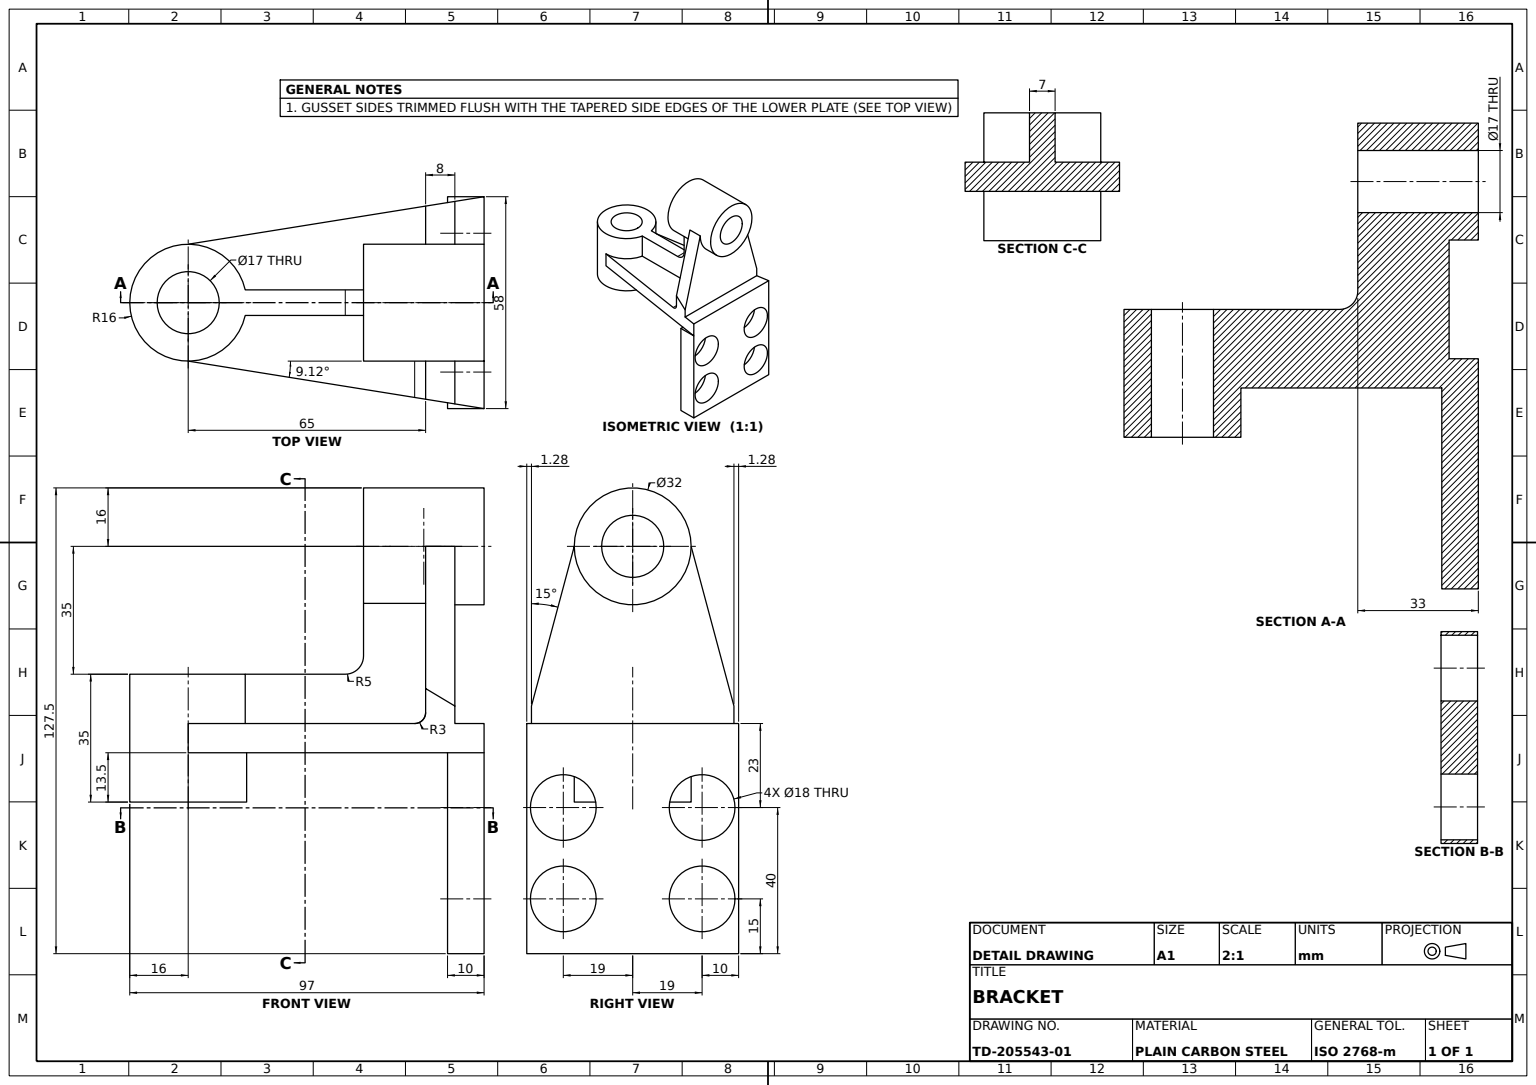
from build123d import *

# Parameters (mm, degrees)
MAIN_BOSS_SKETCH_32_R    = 16
MAIN_BOSS_32_DEPTH       = 17.5
MAIN_BOSS_BORE_SKETCH_R  = 8.5
MAIN_BOSS_BORE_DEPTH     = 57
LOWER_ARM_PLATE_DEPTH    = 4
UPPER_BOSS_SKETCH_R      = 16
UPPER_BOSS_DEPTH         = 33
UPPER_BOSS_BORE_SKETCH_R = 8.5
UPPER_BOSS_BORE_DEPTH    = 38
UPPER_ARM_PLATE_DEPTH    = 8
PLATE_CUT_SET_A_DEPTH    = 38
PLATE_CUT_SET_B_DEPTH    = 38
RIB_DEPTH                = 3.5
RIB_FILLET_R5_R          = 5
ARM_JUNCTION_FILLET_R3_R = 3
GUSSET_SKETCH_W          = 58
GUSSET_SKETCH_H          = 10
GUSSET_DEPTH             = 55
GUSSET_TRIM_SKETCH_R     = 9
GUSSET_TRIM_CUT_DEPTH    = 55


with BuildPart() as part:
    # Main Boss Sketch Ø32 → Main Boss Ø32 (new, symmetric)
    with BuildSketch(Plane(origin=(0, 0, 0), x_dir=(1, 0, 0), z_dir=(0, 1, 0))):
        with Locations(Location((0, 0, 0), (0, 0, 270))):
            Circle(MAIN_BOSS_SKETCH_32_R)
    extrude(amount=MAIN_BOSS_32_DEPTH, both=True)

    # Main Boss Bore Sketch → Main Boss Bore (cut)
    with BuildSketch(Plane(origin=(0, 17.5, 0), x_dir=(1, 0, 0), z_dir=(0, 1, 0))):
        with Locations(Location((0, 0, 0), (0, 0, 270))):
            Circle(MAIN_BOSS_BORE_SKETCH_R)
    extrude(amount=-MAIN_BOSS_BORE_DEPTH, mode=Mode.SUBTRACT)

    # Lower Arm Sketch → Lower Arm Plate (add, symmetric)
    with BuildSketch(Plane(origin=(0, 0, 0), x_dir=(1, 0, 0), z_dir=(0, 1, 0))):
        with BuildLine():
            Line((0, 81), (29, 81))
            Line((29, 81), (16, 0))
            ThreePointArc((16, 0), (0, 16), (-16, 0))
            Line((-16, 0), (-29, 81))
            Line((-29, 81), (0, 81))
        make_face()
    extrude(amount=LOWER_ARM_PLATE_DEPTH, both=True)



with BuildPart() as body_2:
    # Upper Boss Sketch → Upper Boss (new body)
    with BuildSketch(Plane.XY.offset(-48)):
        with Locations((0, 52.5)):
            Circle(UPPER_BOSS_SKETCH_R)
    extrude(amount=-UPPER_BOSS_DEPTH)

    # Upper Boss Bore Sketch → Upper Boss Bore (cut)
    with BuildSketch(Plane.XY.offset(-48)):
        with Locations((0, 52.5)):
            Circle(UPPER_BOSS_BORE_SKETCH_R)
    extrude(amount=-UPPER_BOSS_BORE_DEPTH, mode=Mode.SUBTRACT)


with BuildPart() as part_1:
    add(part.part)

    add(body_2.part)  # Upper Arm Plate merges body 2
    # Upper Arm Sketch → Upper Arm Plate (add)
    with BuildSketch(Plane.XY.offset(-65)):
        with BuildLine():
            Line((-26.431737368, 4), (29, 4))
            Line((29, 4), (16, 52.5))
            ThreePointArc((16, 52.5), (0, 36.5), (-16, 52.5))
            Line((-16, 52.5), (-29, 4))
            Line((-29, 4), (-26.431737368, 4))
        make_face()
    extrude(amount=-UPPER_ARM_PLATE_DEPTH)

    # Plate Cut Set A Sketch → Plate Cut Set A (cut)
    with BuildSketch(Plane.XZ.offset(4)):
        Polygon((27.716049383, -73), (26.432098765, -65), (29, -65), (29, -73), align=None)
    extrude(amount=-PLATE_CUT_SET_A_DEPTH, mode=Mode.SUBTRACT)

    # Plate Cut Set B Sketch → Plate Cut Set B (cut)
    with BuildSketch(Plane.XZ.offset(4)):
        Polygon((-26.432098765, -65), (-29, -65), (-29, -73), (-27.716049383, -73), align=None)
    extrude(amount=-PLATE_CUT_SET_B_DEPTH, mode=Mode.SUBTRACT)

    # Rib Sketch → Rib (add, symmetric)
    with BuildSketch(Plane(origin=(0, 0, 0), x_dir=(0, 0, -1), z_dir=(1, 0, 0))):
        Polygon((48, 17.5), (11.269108444, 17.5), (11.269108444, 4), (65, 4), (65, 40.002332079), (48, 40.002332079), align=None)
    extrude(amount=RIB_DEPTH, both=True)

    # Rib Fillet R5
    rib_fillet_r5_edges = [part_1.edges().sort_by_distance(p)[0] for p in [
        (0, 17.5, -48),
    ]]
    fillet(rib_fillet_r5_edges, radius=RIB_FILLET_R5_R)

    # Arm Junction Fillet R3
    arm_junction_fillet_r3_edges = [part_1.edges().sort_by_distance(p)[0] for p in [
        (14.966049383, 4, -65),
    ]]
    fillet(arm_junction_fillet_r3_edges, radius=ARM_JUNCTION_FILLET_R3_R)

    # Gusset Sketch → Gusset (add)
    with BuildSketch(Plane.XZ.offset(4)):
        with Locations((0, -76)):
            Rectangle(GUSSET_SKETCH_W, GUSSET_SKETCH_H)
    extrude(amount=GUSSET_DEPTH)

    # Gusset Trim Sketch → Gusset Trim Cut (cut)
    with BuildSketch(Plane.XY.offset(-71)):
        with Locations((19, -44)):
            Circle(GUSSET_TRIM_SKETCH_R)
        with Locations((19, -19)):
            Circle(GUSSET_TRIM_SKETCH_R)
        with Locations((-19, -44)):
            Circle(GUSSET_TRIM_SKETCH_R)
        with Locations((-19, -19)):
            Circle(GUSSET_TRIM_SKETCH_R)
    extrude(amount=-GUSSET_TRIM_CUT_DEPTH, mode=Mode.SUBTRACT)


solid = part_1.part
